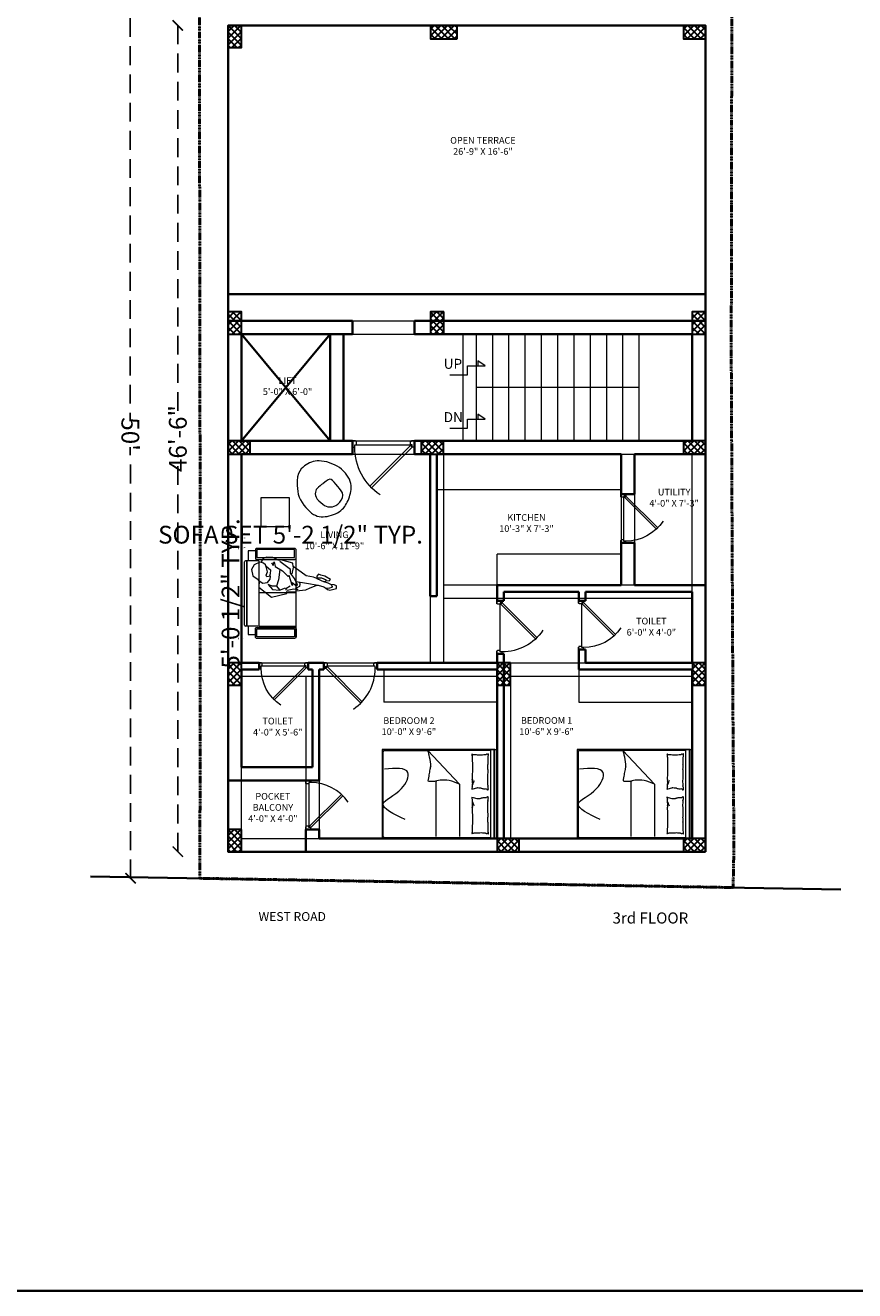
# Model space of a CAD drawing. Units: inches. Extents: x -16911 to -9621, y -48626 to -46270.
# Tile 15 of 20: x -10695 to -10135, y -48626 to -47771. Entities that reach past the tile are written whole.
import ezdxf

# ---------------------------------------------------------------- set-up
doc = ezdxf.new("R2010")
doc.units = ezdxf.units.IN
for name, pattern in [('DASHDOT', [1, 0.5, -0.25, 0, -0.25]), ('DASHED', [19.05, 12.7, -6.35]), ('DOT2', [3.175, 0, -3.175])]:
    doc.linetypes.add(name, pattern=pattern)
for name, color, linetype, lineweight in [('A-ANNO-DIMS', 2, 'Continuous', 13), ('A-ANNO-SYMB', 3, 'Continuous', 13), ('A-ANNO-TEXT', 7, 'Continuous', 18), ('A-AREA-IDEN', 3, 'Continuous', 18), ('A-DOOR', 4, 'Continuous', 18), ('A-FLOR-STRS', 3, 'Continuous', 18), ('A-FURN', 8, 'Continuous', 13), ('A-WALL', 7, 'Continuous', 35), ('C-PROP', 6, 'DASHDOT', 50), ('column', 12, 'Continuous', 30), ('DOOR', 143, 'Continuous', 9), ('EXT BEAM', 132, 'Continuous', 13), ('furniture', 35, 'Continuous', 15), ('Man', 8, 'Continuous', 5), ('S-BEAM', 132, 'Continuous', 25), ('S-COLS', 1, 'Continuous', 30), ('STAIRCASE', 137, 'Continuous', 5)]:
    doc.layers.add(name, color=color, linetype=linetype, lineweight=lineweight)
doc.styles.get("Standard").update_dxf_attribs({"font": 'swissel.ttf'})
doc.styles.add('style9', font='swisscl.ttf', dxfattribs={"height": 12})
doc.dimstyles.new('Dim9', dxfattribs={"dimtxt": 10, "dimasz": 0.199219, "dimexe": 1, "dimexo": 0.5, "dimgap": 1, "dimtad": 0, "dimdec": 1, "dimzin": 0, "dimdsep": 46, "dimlunit": 4, "dimtxsty": 'style9', "dimblk": 'ARCHTICK', "dimcen": 0.09, "dimclrd": 256, "dimclrt": 256, "dimadec": 0, "dimazin": 0, "dimtfac": 1, "dimtdec": 1, "dimtix": 1, "dimtofl": 0, "dimtmove": 1, "dimatfit": 3, "dimfxl": 9, "dimtolj": 1, "dimtzin": 0, "dimlwd": -1, "dimarcsym": 0})

# ---------------------------------------------------------------- blocks, each defined once
blk = doc.blocks.new('Bipman02')
blk.add_lwpolyline([(0.587, -0.067), (0.618, -0.05), (0.652, -0.054), (0.67, -0.038), (0.596, 0.007), (0.544, 0.016), (0.516, 0.03), (0.496, 0.007), (0.492, -0.023), (0.452, -0.006), (0.357, 0.011), (0.292, 0.055), (0.192, 0.129), (0.187, 0.172), (0.031, 0.216), (0.005, 0.207), (-0.069, 0.246), (-0.147, 0.25), (-0.195, 0.233), (-0.225, 0.181), (-0.238, 0.185), (-0.308, 0.15), (-0.343, 0.09), (-0.325, 0.011), (-0.256, -0.037), (-0.247, -0.058), (-0.251, -0.137), (-0.086, -0.263), (0.109, -0.215), (0.109, -0.193), (0.226, -0.197), (0.231, -0.184), (0.352, -0.171), (0.409, -0.145), (0.487, -0.115), (0.509, -0.11), (0.583, -0.132), (0.609, -0.15), (0.63, -0.164), (0.661, -0.176), (0.744, -0.154), (0.748, -0.119), (0.714, -0.105), (0.674, -0.102), (0.639, -0.084)], close=True)
for points in [[(-0.256, -0.045), (-0.199, -0.084), (-0.138, -0.076), (-0.104, -0.032), (-0.099, 0.007), (-0.147, -0.002), (-0.156, 0.016), (-0.138, 0.059), (-0.151, 0.111), (-0.165, 0.15), (-0.191, 0.172), (-0.217, 0.181)], [(-0.086, 0.177), (-0.065, 0.142), (-0.052, 0.19), (-0.039, 0.129), (0.053, 0.072), (0.127, 0.003), (0.135, 0.016), (0.174, -0.106), (0.187, -0.11), (0.179, -0.076), (0.235, -0.119), (0.248, -0.106), (0.209, -0.023), (0.157, 0.042), (0.157, 0.09), (0.018, 0.194)], [(-0.156, 0.133), (-0.099, 0.085), (-0.104, 0.033), (-0.112, 0.007)], [(0.018, 0.09), (0.001, -0.041), (-0.025, -0.123), (-0.078, -0.123), (-0.13, -0.102), (-0.073, -0.167), (0.014, -0.176), (0.092, -0.145), (0.101, -0.176)], [(0.192, 0.116), (0.174, 0.037)], [(-0.025, -0.123), (0.014, -0.171)], [(0.096, -0.154), (0.153, -0.119)], [(0.27, -0.076), (0.274, -0.097), (0.27, -0.128), (0.244, -0.141), (0.222, -0.145), (0.248, -0.163), (0.248, -0.171), (0.2, -0.163), (0.114, -0.18)], [(0.231, -0.063), (0.361, -0.084), (0.509, -0.109)], [(0.492, -0.023), (0.587, -0.067)], [(0.505, -0.015), (0.552, -0.015), (0.613, -0.041)], [(0.678, -0.11), (0.691, -0.128), (0.687, -0.141), (0.657, -0.15), (0.609, -0.154)]]:
    blk.add_lwpolyline(points)
blk = doc.blocks.new('erertety')
at = {"layer": 'furniture', "ltscale": 0.2}
for p, q in [((-17662.13, -45230.66), (-17662.13, -45176.69)), ((-17693.83, -45223.2), (-17693.83, -45184.43)), ((-17685.49, -45183.68), (-17693.08, -45183.68)), ((-17684.74, -45223.2), (-17684.74, -45184.43)), ((-17684.74, -45203.31), (-17662.13, -45203.31)), ((-17685.49, -45223.95), (-17693.08, -45223.95)), ((-17691.58, -45223.95), (-17691.58, -45229.1)), ((-17684.74, -45223.99), (-17662.13, -45223.99)), ((-17684.74, -45224.55), (-17662.13, -45224.55)), ((-17684.74, -45224.55), (-17662.13, -45224.55)), ((-17691.58, -45229.1), (-17687.09, -45229.1))]:
    blk.add_line(p, q, dxfattribs=at)
blk.add_lwpolyline([(-17687.09, -45177.54), (-17691.58, -45177.54), (-17691.58, -45183.68)], dxfattribs=at)
for points in [[(-17662.13, -45182.17), (-17662.13, -45176.97, 0.414214), (-17662.87, -45176.22), (-17686.34, -45176.22, 0.414214), (-17687.09, -45176.97), (-17687.09, -45182.17, 0.414214), (-17686.34, -45182.91), (-17662.87, -45182.91, 0.414214)], [(-17662.13, -45225.47), (-17662.13, -45230.66, -0.414214), (-17662.87, -45231.41), (-17686.34, -45231.41, -0.414214), (-17687.09, -45230.66), (-17687.09, -45225.47, -0.414214), (-17686.34, -45224.72), (-17662.87, -45224.72, -0.414214)]]:
    blk.add_lwpolyline(points, format="xyb", close=True, dxfattribs=at)
for points in [[(-17663.01, -45181.75), (-17663.01, -45176.82), (-17686.21, -45176.82), (-17686.21, -45181.75)], [(-17692.4, -45183.68), (-17692.4, -45223.95), (-17692.4, -45223.95), (-17692.4, -45183.68)], [(-17663.01, -45225.6), (-17663.01, -45230.53), (-17686.21, -45230.53), (-17686.21, -45225.6)]]:
    blk.add_lwpolyline(points, close=True, dxfattribs=at)
for centre, start, end in [((-17693.08, -45184.43), 90, 180), ((-17685.49, -45184.43), 0, 90), ((-17693.08, -45223.2), 180, 270), ((-17685.49, -45223.2), 270, 0)]:
    blk.add_arc(centre, 0.748, start, end, dxfattribs=at)
at = {"layer": 'furniture', "ltscale": 0.2, "xscale": 47.90818138957024, "yscale": 47.90818138957024, "zscale": 47.90818138957024}
blk.add_blockref('Bipman02', (-17673, -45193.44, 0), dxfattribs=at)
blk = doc.blocks.new('rthrty')
at = {"layer": 'furniture'}
blk.add_open_spline([(-17650.3, -45154.53), (-17651.97, -45142.9), (-17645.3, -45136.31), (-17637.11, -45132.37), (-17620.71, -45137.17), (-17612.47, -45149.45), (-17615.73, -45159.71), (-17619.67, -45168.02), (-17632.28, -45172.65), (-17641.84, -45170.43), (-17649.5, -45159.42), (-17650.3, -45154.53)], degree=3, dxfattribs=at)
at = {"layer": 'Man'}
blk.add_open_spline([(-17632.99, -45149.02), (-17629.89, -45146.6), (-17628, -45145.12), (-17623.29, -45151.15), (-17618.06, -45156.77), (-17623.15, -45164.08), (-17628.28, -45165.32), (-17631.61, -45164.6), (-17638.01, -45159.61), (-17638.81, -45154.69), (-17636.9, -45151.81), (-17632.99, -45149.02), (-17632.99, -45149.02)], degree=3, dxfattribs=at)
blk = doc.blocks.new('hjuyuiuyk')
at = {"layer": 'furniture'}
for p, q in [((-19327.49, -39738.98), (-19327.49, -39737.31)), ((-19327.49, -39737.31), (-19267.49, -39737.31, 0)), ((-19327.49, -39746.54), (-19327.49, -39737.31)), ((-19267.49, -39738.5), (-19327.49, -39738.5, 0)), ((-19327.49, -39738.5, 0), (-19327.49, -39814.72, 0)), ((-19327.49, -39738.5), (-19327.49, -39814.72)), ((-19267.49, -39738.5, 0), (-19327.49, -39738.5)), ((-19267.49, -39738.98, 0), (-19327.49, -39738.98)), ((-19268.1, -39741.33), (-19326.9, -39741.33)), ((-19326.9, -39741.33), (-19326.9, -39813.21)), ((-19268.1, -39813.21), (-19268.1, -39741.33)), ((-19267.49, -39737.31, 0), (-19267.49, -39738.98, 0)), ((-19267.49, -39746.54, 0), (-19267.49, -39737.31, 0)), ((-19267.49, -39814.72), (-19267.49, -39738.5)), ((-19267.49, -39814.72, 0), (-19267.49, -39738.5, 0)), ((-19300.88, -39753.22, 0), (-19301.49, -39750.81, 0)), ((-19294.97, -39753.22, 0), (-19294.37, -39750.81, 0)), ((-19300.67, -39754.09, 0), (-19300.88, -39753.22, 0)), ((-19295.19, -39754.09, 0), (-19294.97, -39753.22, 0)), ((-19304.07, -39762.52), (-19326.9, -39783.91)), ((-19304.07, -39762.52), (-19268.82, -39762.52)), ((-19326.9, -39813.21), (-19326.9, -39783.91)), ((-19268.82, -39778.34), (-19306.29, -39778.34)), ((-19327.49, -39814.72, 0), (-19267.49, -39814.72)), ((-19327.49, -39814.72), (-19267.49, -39814.72, 0)), ((-19269.1, -39814.21), (-19325.9, -39814.21)), ((-19325.9, -39814.21), (-19269.1, -39814.21))]:
    blk.add_line(p, q, dxfattribs=at)
for centre, radius, start, end in [((-19324.36, -39743.07, 0), 0.0997, 111.7883, 160.43603), ((-19324.39, -39743.06, 0), 0.0676, 160.43603, 281.89306), ((-19324.12, -39743.66, 0), 0.732, 94.30254, 111.7883), ((-19324.35, -39743.25, 0), 0.125, 21.9904, 101.89306), ((-19323.34, -39743.89, 0), 0.956, 158.57902, 188.13348), ((-19324.65, -39743.37, 0), 0.455, 338.57902, 21.9904), ((-19324.11, -39743.77, 0), 0.842, 59.34875, 94.30254), ((-19322.88, -39741.69, 0), 1.57, 239.34875, 264.74081), ((-19319.6, -39692.5, 0), 50.87, 266.13994, 268.60024), ((-19319.84, -39713.09, 0), 30.28, 268.09211, 271.28082), ((-19320.24, -39695.07, 0), 48.31, 271.28082, 273.40341), ((-19316.15, -39763.89, 0), 20.63, 90.1553, 93.40341), ((-19316.09, -39783.15, 0), 39.89, 86.99024, 90.1553), ((-19305.86, -39588.51, 0), 155.02, 266.99024, 268.59569), ((-19305.42, -39570.46, 0), 173.07, 268.59569, 270), ((-19305.42, -39718.38, 0), 25.15, 270, 273.68415), ((-19304.03, -39739.9, 0), 3.58, 273.68415, 287.19507), ((-19300.46, -39751.46, 0), 8.51, 98.43719, 107.19507), ((-19301.02, -39747.69, 0), 4.7, 90, 98.43719), ((-19301.12, -39743.14, 0), 0.997, 274.40021, 333.41948), ((-19301.02, -39745.63, 0), 2.64, 78.72762, 90), ((-19300.58, -39743.42, 0), 0.383, 333.41948, 78.72762), ((-19295.28, -39743.42, 0), 0.383, 101.27238, 206.58052), ((-19294.73, -39743.14, 0), 0.997, 206.58052, 265.59979), ((-19294.84, -39745.63, 0), 2.64, 90, 101.27238), ((-19294.84, -39747.69, 0), 4.7, 81.56281, 90), ((-19295.39, -39751.46, 0), 8.51, 72.80493, 81.56281), ((-19291.82, -39739.9, 0), 3.58, 252.80493, 266.31585), ((-19290.43, -39718.38, 0), 25.15, 266.31585, 270), ((-19290.43, -39570.46, 0), 173.07, 270, 271.40431), ((-19289.99, -39588.51, 0), 155.02, 271.40431, 273.00976), ((-19279.76, -39783.15, 0), 39.89, 89.8447, 93.00976), ((-19279.7, -39763.89, 0), 20.63, 86.59659, 89.8447), ((-19275.61, -39695.07, 0), 48.31, 266.59659, 268.71918), ((-19276.02, -39713.09, 0), 30.28, 268.71918, 271.90789), ((-19276.73, -39645.13, 0), 98.25, 271.00686, 272.7772), ((-19272.12, -39741.69, 0), 1.57, 275.25919, 300.65125), ((-19270.89, -39743.77, 0), 0.842, 85.69746, 120.65125), ((-19270.88, -39743.66, 0), 0.732, 68.2117, 85.69746), ((-19270.35, -39743.37, 0), 0.455, 158.0096, 201.42098), ((-19270.65, -39743.25, 0), 0.125, 78.10694, 158.0096), ((-19271.66, -39743.89, 0), 0.956, 351.86652, 21.42098), ((-19270.61, -39743.06, 0), 0.0676, 258.10694, 19.56397), ((-19270.64, -39743.07, 0), 0.0997, 19.56397, 68.2117), ((-19317.18, -39743.01, 0), 7.17, 188.13348, 192.10946), ((-19329.85, -39745.73, 0), 5.78, 7.6809, 12.10946), ((-19350.51, -39748.51, 0), 26.62, 3.36875, 7.6809), ((-19720.99, -39728.47, 0), 397.61, 356.49514, 356.94504), ((-19363.7, -39747.54, 0), 39.81, 356.94504, 358.36691), ((-19343.69, -39748.11, 0), 19.79, 358.36691, 3.36875), ((-19299.57, -39750.33, 0), 1.97, 177.33512, 194.04519), ((-19282.35, -39751.13, 0), 19.21, 171.99495, 177.33512), ((-19292.22, -39749.75, 0), 9.25, 167.80162, 171.99495), ((-19326.4, -39742.36, 0), 25.72, 347.80162, 350.31563), ((-19315.3, -39745.68, 0), 14.34, 360, 6.23236), ((-19306.91, -39745.68, 0), 5.95, 350.31563, 360), ((-19280.55, -39745.68, 0), 14.34, 173.76764, 180), ((-19288.94, -39745.68, 0), 5.95, 180, 189.68437), ((-19269.45, -39742.36, 0), 25.72, 189.68437, 192.19838), ((-19303.63, -39749.75, 0), 9.25, 8.00505, 12.19838), ((-19313.5, -39751.13, 0), 19.21, 2.66488, 8.00505), ((-19296.28, -39750.33, 0), 1.97, 345.95481, 2.66488), ((-19251.31, -39748.11, 0), 19.79, 176.63125, 181.63309), ((-19231.3, -39747.54, 0), 39.81, 181.63309, 183.05496), ((-19244.49, -39748.51, 0), 26.62, 172.3191, 176.63125), ((-18874.01, -39728.47, 0), 397.61, 183.05496, 183.50486), ((-19265.15, -39745.73, 0), 5.78, 167.89054, 172.3191), ((-19277.82, -39743.01, 0), 7.17, 347.89054, 351.86652), ((-19323.69, -39753.93, 0), 0.564, 170.00164, 196.69777), ((-19333.47, -39752.21, 0), 9.37, 350.00164, 356.49514), ((-19324.19, -39754.08, 0), 0.0385, 196.69777, 277.12039), ((-19324.51, -39751.59, 0), 2.55, 277.12039, 286.22115), ((-19324.42, -39751.9, 0), 2.23, 286.22115, 297.44392), ((-19322.81, -39754.99, 0), 1.25, 102.44799, 117.44392), ((-19322.32, -39757.22, 0), 3.54, 93.57397, 102.44799), ((-19318.44, -39837.61, 0), 84.03, 90.97549, 92.79548), ((-19315.55, -39952.16, 0), 198.61, 89.44614, 91.24735), ((-19314.9, -39885.06, 0), 131.51, 87.23256, 89.44614), ((-19310.57, -39795.48, 0), 41.81, 85.40123, 87.23256), ((-19304.32, -39717.78, 0), 36.14, 265.40123, 267.37117), ((-19297.32, -39733.09, 0), 21.54, 244.68893, 246.51559), ((-19305.66, -39747.05, 0), 6.83, 267.37117, 281.48268), ((-19297.32, -39733.09, 0), 21.54, 246.51559, 248.34226), ((-19297.32, -39733.09, 0), 21.54, 248.34226, 250.57202), ((-19297.32, -39733.09, 0), 21.54, 250.57202, 252.80178), ((-19303.46, -39757.91, 0), 4.25, 83.56595, 101.48268), ((-19303.37, -39757.16, 0), 3.49, 72.61359, 83.56595), ((-19300.33, -39747.43, 0), 6.7, 252.61359, 260.5159), ((-19300.13, -39746.25, 0), 7.9, 260.5159, 265.91706), ((-19300.69, -39754.1, 0), 0.0267, 265.91706, 14.04494), ((-19295.16, -39754.1, 0), 0.0267, 165.95506, 274.08294), ((-19295.72, -39746.25, 0), 7.9, 274.08294, 279.4841), ((-19295.52, -39747.43, 0), 6.7, 279.4841, 287.38641), ((-19292.48, -39757.16, 0), 3.49, 96.43405, 107.38641), ((-19292.39, -39757.91, 0), 4.25, 78.51732, 96.43405), ((-19298.54, -39733.09, 0), 21.54, 287.19822, 289.42798), ((-19290.19, -39747.05, 0), 6.83, 258.51732, 272.62883), ((-19298.54, -39733.09, 0), 21.54, 289.42798, 291.65774), ((-19298.54, -39733.09, 0), 21.54, 291.65774, 293.48441), ((-19298.54, -39733.09, 0), 21.54, 293.48441, 295.31107), ((-19291.53, -39717.78, 0), 36.14, 272.62883, 274.59877), ((-19285.28, -39795.48, 0), 41.81, 92.76744, 94.59877), ((-19280.95, -39885.06, 0), 131.51, 90.55386, 92.76744), ((-19280.3, -39952.16, 0), 198.61, 88.75265, 90.55386), ((-19277.1, -39805.01, 0), 51.42, 86.42603, 88.75265), ((-19274.68, -39799.75, 0), 46.07, 86.55746, 89.01709), ((-19272.19, -39754.99, 0), 1.25, 62.55608, 77.55201), ((-19270.58, -39751.9, 0), 2.23, 242.55608, 253.77885), ((-19270.49, -39751.59, 0), 2.55, 253.77885, 262.87961), ((-19261.53, -39752.21, 0), 9.37, 183.50486, 189.99836), ((-19270.81, -39754.08, 0), 0.0385, 262.87961, 343.30223), ((-19271.31, -39753.93, 0), 0.564, 343.30223, 9.99836), ((-19279.47, -39774.89), 27.53, 153.30845, 168.74227), ((-19287.94, -39773.2), 18.89, 168.74227, 187.39945), ((-19242.78, -39767.34), 64.43, 187.39945, 189.27191), ((-19333.07, -39782.08), 27.05, 6.38169, 9.27191), ((-19306.77, -39846.83), 66.07, 105.93519, 107.73639), ((-19318.41, -39806.06), 23.67, 102.92554, 105.93519), ((-19287.64, -39956.87), 177.57, 99.72434, 101.71957), ((-19317.24, -39783.9), 2.09, 82.26962, 100.72756), ((-19317.9, -39788.76), 6.99, 76.8096, 82.26962), ((-19295.64, -39693.77), 90.57, 256.8096, 258.32586), ((-19295.11, -39691.23), 93.17, 258.32586, 260.50498), ((-19288.03, -39648.9), 136.08, 260.50498, 262.308), ((-19336.71, -39780.62), 30.63, 354.11415, 359.23133), ((-19321.79, -39780.82), 15.7, 359.23133, 6.38169), ((-19325.9, -39813.21), 1, 180, 270), ((-19269.1, -39813.21), 1, 270, 0)]:
    blk.add_arc(centre, radius, start, end, dxfattribs=at)
blk.add_open_spline([(-19280.24, -39799.21), (-19283.87, -39806.94), (-19290.73, -39821.55), (-19298.08, -39801.09), (-19315.85, -39793.47), (-19314.86, -39805.92), (-19314.29, -39813.13)], degree=3, knots=[0, 0, 0, 0, 18.167809, 34.338432, 45.972904, 61.997799, 61.997799, 61.997799, 61.997799], dxfattribs=at)
blk = doc.blocks.new('A$C1C9D3E54')
at = {"layer": 'DOOR'}
blk.add_line((18676.53, 5780.72), (18710.53, 5780.72), dxfattribs=at)
blk.add_lwpolyline([(18685.01, 5806.62), (18710.47, 5781.16), (18711.53, 5782.22), (18686.07, 5807.68), (18685.01, 5806.62)], dxfattribs=at)
blk.add_lwpolyline([(18674.03, 5778.22), (18676.03, 5778.22), (18674.03, 5778.22), (18674.03, 5782.22), (18675.53, 5782.22), (18675.53, 5780.72), (18676.53, 5780.72), (18676.53, 5778.72), (18676.41, 5778.72), (18676.41, 5778.6, -0.414214), (18676.16, 5778.35), (18676.03, 5778.35), (18676.03, 5778.22)], format="xyb", dxfattribs=at)
blk.add_lwpolyline([(18713.03, 5782.22), (18711.53, 5782.22), (18711.53, 5780.72), (18710.53, 5780.72), (18710.53, 5778.72), (18710.66, 5778.72), (18710.66, 5778.6, 0.414214), (18710.91, 5778.35), (18711.03, 5778.35), (18711.03, 5778.22), (18713.03, 5778.22), (18711.03, 5778.22), (18713.03, 5778.22), (18713.03, 5782.22)], format="xyb", close=True, dxfattribs=at)
blk.add_arc((18711.53, 5782.22), 36, 124.03362, 180, dxfattribs=at)
blk = doc.blocks.new('_ArchTick')
at = {"color": 0, "linetype": 'ByBlock', "const_width": 0.15}
blk.add_lwpolyline([(-0.5, -0.5), (0.5, 0.5)], dxfattribs=at)
blk = doc.blocks.new('*D24')
at = {"layer": 'A-ANNO-DIMS', "color": 0, "linetype": 'DOT2', "lineweight": -2, "transparency": 16777216}
for p, q in [((-10623.85, -47747.46), (-10625.04, -47747.46)), ((-10623.49, -48347.46), (-10624.67, -48347.46))]:
    blk.add_line(p, q, dxfattribs=at)
at = {"layer": 'A-ANNO-DIMS', "color": 0, "linetype": 'DASHED', "lineweight": 25, "transparency": 16777216}
for p, q in [((-10624.04, -47747.46), (-10623.86, -48038.62)), ((-10623.67, -48347.46), (-10623.85, -48056.3))]:
    blk.add_line(p, q, dxfattribs=at)
at = {"layer": 'Defpoints', "color": 0, "transparency": 16777216}
for p in [(-10624.04, -47747.46), (-10605.22, -47747.45), (-10604.86, -48347.45)]:
    blk.add_point(p, dxfattribs=at)
at = {"layer": 'A-ANNO-DIMS', "color": 0, "lineweight": 25, "transparency": 16777216, "xscale": 7, "yscale": 7, "zscale": 7}
for p, rotation in [((-10624.04, -47747.46), 90.0346840750536), ((-10623.67, -48347.46), 270.0346840750536)]:
    blk.add_blockref('_ArchTick', p, dxfattribs=dict(at, rotation=rotation))
at = {"layer": 'A-ANNO-DIMS', "color": 0, "transparency": 16777216, "insert": (-10623.85, -48047.46), "char_height": 12, "attachment_point": 5, "rotation": 270.03468, "style": 'style9'}
blk.add_mtext("\\A1;50'", dxfattribs=at)
blk = doc.blocks.new('*D26')
at = {"layer": 'A-ANNO-DIMS', "color": 0, "linetype": 'DOT2', "lineweight": -2, "transparency": 16777216}
for p, q in [((-10591.56, -47771.49), (-10592.75, -47771.49)), ((-10591.56, -48329.45), (-10592.75, -48329.45))]:
    blk.add_line(p, q, dxfattribs=at)
at = {"layer": 'A-ANNO-DIMS', "color": 0, "linetype": 'DASHED', "lineweight": 25, "transparency": 16777216}
for p, q in [((-10591.75, -47771.49), (-10591.75, -48032.84)), ((-10591.75, -48329.45), (-10591.75, -48068.11))]:
    blk.add_line(p, q, dxfattribs=at)
at = {"layer": 'Defpoints', "color": 0, "transparency": 16777216}
for p in [(-10557.82, -47771.49), (-10591.75, -48329.45), (-10557.82, -48329.45)]:
    blk.add_point(p, dxfattribs=at)
at = {"layer": 'A-ANNO-DIMS', "color": 0, "lineweight": 25, "transparency": 16777216, "xscale": 7, "yscale": 7, "zscale": 7}
for p, rotation in [((-10591.75, -47771.49), 90), ((-10591.75, -48329.45), 270)]:
    blk.add_blockref('_ArchTick', p, dxfattribs=dict(at, rotation=rotation))
at = {"layer": 'A-ANNO-DIMS', "color": 0, "transparency": 16777216, "insert": (-10591.75, -48050.47), "char_height": 12, "attachment_point": 5, "rotation": 90, "style": 'style9'}
blk.add_mtext('\\A1;46\'-6"', dxfattribs=at)
blk = doc.blocks.new('THYHYTJ')
at = {"layer": 'STAIRCASE', "ltscale": 10}
for p, q in [((-7981.18, -46346.18), (-7984.62, -46351.1)), ((-7981.18, -46358.18), (-7981.18, -46346.18)), ((-7984.62, -46351.1), (-7981.18, -46351.1)), ((-7975.18, -46358.18), (-7981.18, -46358.18)), ((-7975.18, -46370.18), (-7975.18, -46358.18))]:
    blk.add_line(p, q, dxfattribs=at)
blk = doc.blocks.new('COLUMNS')
at = {"layer": 'column'}
h = blk.add_hatch(dxfattribs=at)
h.set_pattern_fill('ANSI37', color=256, angle=-720)
h.set_pattern_definition([(45, (21703.4588, -104481.6704), (-2.24506403, 2.24506403), []), (135, (21703.4588, -104481.6704), (-2.24506403, -2.24506403), [])])
h.paths.add_polyline_path([(-12061.47, -46401.86), (-12052.47, -46401.86), (-12052.47, -46386.86), (-12061.47, -46386.86)])
h = blk.add_hatch(dxfattribs=at)
h.set_pattern_fill('ANSI37', color=256, angle=-810)
h.set_pattern_definition([(315, (-70004.5392, -80151.7886), (2.24506403, 2.24506403), []), (45, (-70004.5392, -80151.7886), (-2.24506403, 2.24506403), [])])
h.paths.add_polyline_path([(-11924.72, -46386.86), (-11924.72, -46395.86), (-11906.72, -46395.86), (-11906.72, -46386.86)])
h = blk.add_hatch(dxfattribs=at)
h.set_pattern_fill('ANSI37', color=256, angle=-810)
h.set_pattern_definition([(315, (-69833.7395, -80151.7886), (2.24506403, 2.24506403), []), (45, (-69833.7395, -80151.7886), (-2.24506403, 2.24506403), [])])
h.paths.add_polyline_path([(-11753.92, -46386.86), (-11753.92, -46395.86), (-11738.92, -46395.86), (-11738.92, -46386.86)])
h = blk.add_hatch(dxfattribs=at)
h.set_pattern_fill('ANSI37', color=256, angle=-900)
h.set_pattern_definition([(225, (-45817.4075, 11499.4594), (2.24506403, -2.24506403), []), (315, (-45817.4075, 11499.4594), (2.24506403, 2.24506403), [])])
h.paths.add_polyline_path([(-12052.47, -46580.36), (-12061.47, -46580.36), (-12061.47, -46595.36), (-12052.47, -46595.36)])
h = blk.add_hatch(dxfattribs=at)
h.set_pattern_fill('ANSI37', color=256, angle=-720)
h.set_pattern_definition([(45, (21840.2088, -104675.1704), (-2.24506403, 2.24506403), []), (135, (21840.2088, -104675.1704), (-2.24506403, -2.24506403), [])])
h.paths.add_polyline_path([(-11924.72, -46595.36), (-11915.72, -46595.36), (-11915.72, -46580.36), (-11924.72, -46580.36)])
h = blk.add_hatch(dxfattribs=at)
h.set_pattern_fill('ANSI37', color=256, angle=-900)
h.set_pattern_definition([(225, (-45503.8578, 11499.4594), (2.24506403, -2.24506403), []), (315, (-45503.8578, 11499.4594), (2.24506403, 2.24506403), [])])
h.paths.add_polyline_path([(-11738.92, -46580.36), (-11747.92, -46580.36), (-11747.92, -46595.36), (-11738.92, -46595.36)])
h = blk.add_hatch(dxfattribs=at)
h.set_pattern_fill('ANSI37', color=256, angle=-810)
h.set_pattern_definition([(315, (-70141.2892, -80432.2886), (2.24506403, 2.24506403), []), (45, (-70141.2892, -80432.2886), (-2.24506403, 2.24506403), [])])
h.paths.add_polyline_path([(-12061.47, -46667.36), (-12061.47, -46676.36), (-12046.47, -46676.36), (-12046.47, -46667.36)])
h = blk.add_hatch(dxfattribs=at)
h.set_pattern_fill('ANSI37', color=256, angle=-810)
h.set_pattern_definition([(315, (-70010.7892, -80432.2886), (2.24506403, 2.24506403), []), (45, (-70010.7892, -80432.2886), (-2.24506403, 2.24506403), [])])
h.paths.add_polyline_path([(-11930.97, -46667.36), (-11930.97, -46676.36), (-11915.97, -46676.36), (-11915.97, -46667.36)])
h = blk.add_hatch(dxfattribs=at)
h.set_pattern_fill('ANSI37', color=256, angle=-810)
h.set_pattern_definition([(315, (-69833.7395, -80432.2886), (2.24506403, 2.24506403), []), (45, (-69833.7395, -80432.2886), (-2.24506403, 2.24506403), [])])
h.paths.add_polyline_path([(-11753.92, -46667.36), (-11753.92, -46676.36), (-11738.92, -46676.36), (-11738.92, -46667.36)])
h = blk.add_hatch(dxfattribs=at)
h.set_pattern_fill('ANSI37', color=256, angle=-540)
h.set_pattern_definition([(225, (-45817.4075, 11262.5055), (2.24506403, -2.24506403), []), (315, (-45817.4075, 11262.5055), (2.24506403, 2.24506403), [])])
h.paths.add_polyline_path([(-12052.47, -46817.31), (-12061.47, -46817.31), (-12061.47, -46832.31), (-12052.47, -46832.31)])
h = blk.add_hatch(dxfattribs=at)
h.set_pattern_fill('ANSI37', color=256, angle=-720)
h.set_pattern_definition([(45, (21885.2088, -104912.1242), (-2.24506403, 2.24506403), []), (135, (21885.2088, -104912.1242), (-2.24506403, -2.24506403), [])])
h.paths.add_polyline_path([(-11879.72, -46832.31), (-11870.72, -46832.31), (-11870.72, -46817.31), (-11879.72, -46817.31)])
h = blk.add_hatch(dxfattribs=at)
h.set_pattern_fill('ANSI37', color=256, angle=-720)
h.set_pattern_definition([(45, (22017.1023, -104912.1242), (-2.24506403, 2.24506403), []), (135, (22017.1023, -104912.1242), (-2.24506403, -2.24506403), [])])
h.paths.add_polyline_path([(-11747.83, -46832.31), (-11738.83, -46832.31), (-11738.83, -46817.31), (-11747.83, -46817.31)])
h = blk.add_hatch(dxfattribs=at)
h.set_pattern_fill('ANSI37', color=256, angle=-720)
h.set_pattern_definition([(45, (21703.4588, -105024.6242), (-2.24506403, 2.24506403), []), (135, (21703.4588, -105024.6242), (-2.24506403, -2.24506403), [])])
h.paths.add_polyline_path([(-12061.47, -46944.81), (-12052.47, -46944.81), (-12052.47, -46929.81), (-12061.47, -46929.81)])
h = blk.add_hatch(dxfattribs=at)
h.set_pattern_fill('ANSI37', color=256, angle=-810)
h.set_pattern_definition([(315, (-69959.5392, -80700.7425), (2.24506403, 2.24506403), []), (45, (-69959.5392, -80700.7425), (-2.24506403, 2.24506403), [])])
h.paths.add_polyline_path([(-11879.72, -46935.81), (-11879.72, -46944.81), (-11864.72, -46944.81), (-11864.72, -46935.81)])
h = blk.add_hatch(dxfattribs=at)
h.set_pattern_fill('ANSI37', color=256, angle=-810)
h.set_pattern_definition([(315, (-69833.7395, -80700.7425), (2.24506403, 2.24506403), []), (45, (-69833.7395, -80700.7425), (-2.24506403, 2.24506403), [])])
h.paths.add_polyline_path([(-11753.92, -46935.81), (-11753.92, -46944.81), (-11738.92, -46944.81), (-11738.92, -46935.81)])
at = {"layer": 'column', "ltscale": 0.05}
for points in [[(-12052.47, -46386.86), (-12061.47, -46386.86), (-12061.47, -46401.86), (-12052.47, -46401.86)], [(-11906.72, -46395.86), (-11906.72, -46386.86), (-11924.72, -46386.86), (-11924.72, -46395.86)], [(-11738.92, -46395.86), (-11738.92, -46386.86), (-11753.92, -46386.86), (-11753.92, -46395.86)], [(-12061.47, -46595.36), (-12052.47, -46595.36), (-12052.47, -46580.36), (-12061.47, -46580.36)], [(-11915.72, -46580.36), (-11924.72, -46580.36), (-11924.72, -46595.36), (-11915.72, -46595.36)], [(-11747.92, -46595.36), (-11738.92, -46595.36), (-11738.92, -46580.36), (-11747.92, -46580.36)], [(-12046.47, -46676.36), (-12046.47, -46667.36), (-12061.47, -46667.36), (-12061.47, -46676.36)], [(-11915.97, -46676.36), (-11915.97, -46667.36), (-11930.97, -46667.36), (-11930.97, -46676.36)], [(-11738.92, -46676.36), (-11738.92, -46667.36), (-11753.92, -46667.36), (-11753.92, -46676.36)], [(-12061.47, -46832.31), (-12052.47, -46832.31), (-12052.47, -46817.31), (-12061.47, -46817.31)], [(-11870.72, -46817.31), (-11879.72, -46817.31), (-11879.72, -46832.31), (-11870.72, -46832.31)], [(-11738.83, -46817.31), (-11747.83, -46817.31), (-11747.83, -46832.31), (-11738.83, -46832.31)], [(-12052.47, -46929.81), (-12061.47, -46929.81), (-12061.47, -46944.81), (-12052.47, -46944.81)], [(-11864.72, -46944.81), (-11864.72, -46935.81), (-11879.72, -46935.81), (-11879.72, -46944.81)], [(-11738.92, -46944.81), (-11738.92, -46935.81), (-11753.92, -46935.81), (-11753.92, -46944.81)]]:
    blk.add_lwpolyline(points, close=True, dxfattribs=at)
blk = doc.blocks.new('3RD ROOF BEAMS')
at = {"layer": 'EXT BEAM'}
for p, q in [((-11461.47, -46586.36), (-11324.72, -46586.36)), ((-11461.47, -46944.81), (-11461.47, -46586.36)), ((-11320.47, -46586.36), (-11138.92, -46586.36)), ((-11138.92, -46944.81), (-11138.92, -46586.36)), ((-11452.47, -46595.36), (-11324.72, -46595.36)), ((-11392.47, -46595.36), (-11392.47, -46667.36)), ((-11383.47, -46595.36), (-11383.47, -46667.36)), ((-11320.47, -46595.36), (-11147.92, -46595.36)), ((-11302.92, -46595.36), (-11302.92, -46667.36)), ((-11293.92, -46595.36), (-11293.92, -46667.36)), ((-11147.92, -46667.36), (-11147.92, -46595.36)), ((-11446.47, -46667.36), (-11335.47, -46667.36)), ((-11320.47, -46667.36), (-11138.92, -46667.36)), ((-11452.47, -46817.31), (-11452.47, -46676.36)), ((-11446.47, -46676.36), (-11335.47, -46676.36)), ((-11324.97, -46676.36), (-11324.97, -46817.31)), ((-11320.47, -46676.36), (-11138.92, -46676.36)), ((-11315.97, -46676.36), (-11315.97, -46817.31)), ((-11195.92, -46676.36), (-11195.92, -46764.81)), ((-11186.92, -46676.36), (-11186.92, -46764.81)), ((-11147.92, -46817.31), (-11147.92, -46676.36)), ((-11147.92, -46764.81), (-11315.97, -46764.81)), ((-11147.92, -46773.81), (-11315.97, -46773.81)), ((-11452.47, -46817.31), (-11147.92, -46817.31)), ((-11452.47, -46826.31), (-11279.72, -46826.31)), ((-11452.47, -46944.81), (-11452.47, -46826.31)), ((-11408.97, -46826.31), (-11408.97, -46935.81)), ((-11399.97, -46826.31), (-11399.97, -46935.81)), ((-11279.72, -46826.31), (-11279.72, -46935.81)), ((-11270.72, -46826.31), (-11147.92, -46826.31)), ((-11270.72, -46826.31), (-11270.72, -46935.81)), ((-11147.92, -46935.81), (-11147.92, -46826.31)), ((-11452.47, -46935.81), (-11279.72, -46935.81)), ((-11270.72, -46935.81), (-11147.92, -46935.81)), ((-11461.47, -46944.81), (-11138.92, -46944.81))]:
    blk.add_line(p, q, dxfattribs=at)
blk = doc.blocks.new('*D73')
at = {"layer": 'A-ANNO-DIMS', "linetype": 'DASHED', "transparency": 16777216}
for p, q in [((-10546.8, -48115.39), (-10547, -48115.39)), ((-10484.48, -48115.39), (-10484.28, -48115.39))]:
    blk.add_line(p, q, dxfattribs=at)
at = {"layer": 'A-ANNO-DIMS', "color": 0, "linetype": 'DOT2', "lineweight": -2, "transparency": 16777216}
for p, q in [((-10546.8, -48124.24), (-10546.8, -48114.39)), ((-10484.48, -48124.24), (-10484.48, -48114.39))]:
    blk.add_line(p, q, dxfattribs=at)
at = {"layer": 'Defpoints', "color": 0, "transparency": 16777216}
for p in [(-10484.48, -48115.39), (-10546.8, -48124.74), (-10484.48, -48124.74)]:
    blk.add_point(p, dxfattribs=at)
at = {"layer": 'A-ANNO-DIMS', "transparency": 16777216, "xscale": 0.19921875, "yscale": 0.19921875, "zscale": 0.19921875}
blk.add_blockref('_ArchTick', (-10546.8, -48115.39), dxfattribs=at)
at = {"layer": 'A-ANNO-DIMS', "transparency": 16777216, "xscale": 0.19921875, "yscale": 0.19921875, "zscale": 0.19921875, "rotation": 180}
blk.add_blockref('_ArchTick', (-10484.48, -48115.39), dxfattribs=at)
at = {"layer": 'A-ANNO-DIMS', "transparency": 16777216, "insert": (-10515.64, -48115.39), "char_height": 12, "attachment_point": 5, "style": 'style9'}
blk.add_mtext('\\A1;SOFA SET 5\'-2 1/2" TYP.', dxfattribs=at)
blk = doc.blocks.new('*D74')
at = {"layer": 'A-ANNO-DIMS', "color": 0, "linetype": 'DOT2', "lineweight": -2, "transparency": 16777216}
for p, q in [((-10547.3, -48124.74), (-10557.15, -48124.74)), ((-10547.3, -48185.44), (-10557.15, -48185.44))]:
    blk.add_line(p, q, dxfattribs=at)
at = {"layer": 'A-ANNO-DIMS', "linetype": 'DASHED', "transparency": 16777216}
for p, q in [((-10556.15, -48124.74), (-10556.15, -48124.54)), ((-10556.15, -48185.44), (-10556.15, -48185.64))]:
    blk.add_line(p, q, dxfattribs=at)
at = {"layer": 'Defpoints', "color": 0, "transparency": 16777216}
for p in [(-10556.15, -48124.74), (-10546.8, -48124.74), (-10546.8, -48185.44)]:
    blk.add_point(p, dxfattribs=at)
at = {"layer": 'A-ANNO-DIMS', "transparency": 16777216, "xscale": 0.19921875, "yscale": 0.19921875, "zscale": 0.19921875}
for p, rotation in [((-10556.15, -48124.74), 270), ((-10556.15, -48185.44), 90)]:
    blk.add_blockref('_ArchTick', p, dxfattribs=dict(at, rotation=rotation))
at = {"layer": 'A-ANNO-DIMS', "transparency": 16777216, "insert": (-10556.15, -48155.09), "char_height": 12, "attachment_point": 5, "rotation": 90, "style": 'style9'}
blk.add_mtext('\\A1;5\'-0 1/2" TYP.', dxfattribs=at)

msp = doc.modelspace()

# ---------------------------------------------------------------- linework, layer by layer
at = {"layer": 'A-FLOR-STRS', "ltscale": 10}
for p, q in [((-10390.274, -47979.994), (-10390.274, -48051.994)), ((-10379.274, -47979.994), (-10379.274, -48051.994)), ((-10368.274, -47979.994), (-10368.274, -48051.994)), ((-10357.274, -47979.994), (-10357.274, -48051.994)), ((-10346.274, -47979.994), (-10346.274, -48051.994)), ((-10335.274, -47979.994), (-10335.274, -48051.994)), ((-10324.274, -47979.994), (-10324.274, -48051.994)), ((-10313.274, -47979.994), (-10313.274, -48051.994)), ((-10302.274, -47979.994), (-10302.274, -48051.994)), ((-10291.274, -47979.994), (-10291.274, -48051.994)), ((-10280.274, -47979.994), (-10280.274, -48051.994)), ((-10280.274, -48015.994), (-10390.274, -48015.994))]:
    msp.add_line(p, q, dxfattribs=at)
at = {"layer": 'A-FURN', "ltscale": 0.2}
for p, q in [((-10292.274, -48084.994), (-10416.824, -48084.994)), ((-10292.274, -48128.448), (-10376.074, -48128.448)), ((-10376.074, -48149.448), (-10376.074, -48128.448)), ((-10452.574, -48206.448, 0), (-10452.574, -48228.448, 0)), ((-10320.774, -48206.448), (-10320.774, -48228.448)), ((-10376.074, -48228.448), (-10452.574, -48228.448)), ((-10320.774, -48228.448), (-10244.274, -48228.448))]:
    msp.add_line(p, q, dxfattribs=at)
at = {"layer": 'A-FURN'}
msp.add_lwpolyline([(-10516.228, -48090.39), (-10535.588, -48090.39), (-10535.588, -48109.75), (-10516.228, -48109.75)], close=True, dxfattribs=at)
at = {"layer": 'A-WALL'}
for p, q in [((-10235.274, -47771.494), (-10557.824, -47771.494)), ((-10557.824, -47970.994), (-10557.824, -47771.494)), ((-10235.274, -47771.494), (-10235.274, -47970.994)), ((-10557.824, -47952.994), (-10235.274, -47952.994)), ((-10557.824, -48281.448), (-10557.824, -47970.994)), ((-10473.824, -47970.994), (-10557.824, -47970.994)), ((-10473.824, -47979.994), (-10473.824, -47970.994)), ((-10235.274, -47970.994), (-10431.824, -47970.994)), ((-10431.824, -47979.994), (-10431.824, -47970.994)), ((-10235.274, -47970.994), (-10235.274, -48060.994)), ((-10548.824, -48051.994), (-10548.824, -47979.994)), ((-10473.824, -47979.994), (-10548.824, -47979.994)), ((-10548.824, -47979.994), (-10488.824, -48051.994)), ((-10548.824, -48051.994), (-10488.824, -47979.994)), ((-10488.824, -48051.994), (-10488.824, -47979.994)), ((-10479.824, -48051.994), (-10479.824, -47979.994)), ((-10244.274, -47979.994), (-10431.824, -47979.994)), ((-10244.274, -47979.994), (-10244.274, -48051.994)), ((-10473.824, -48051.994), (-10548.824, -48051.994)), ((-10473.824, -48060.994), (-10473.824, -48051.994)), ((-10244.274, -48051.994), (-10431.824, -48051.994)), ((-10431.824, -48060.994), (-10431.824, -48051.994)), ((-10548.824, -48201.948), (-10548.824, -48060.994)), ((-10473.824, -48060.994), (-10548.824, -48060.994)), ((-10421.324, -48060.994), (-10431.824, -48060.994)), ((-10421.324, -48060.994), (-10421.324, -48156.994)), ((-10292.274, -48060.994), (-10416.824, -48060.994)), ((-10416.824, -48060.994), (-10416.824, -48156.994)), ((-10292.274, -48060.994), (-10292.274, -48087.994)), ((-10235.274, -48060.994), (-10283.274, -48060.994)), ((-10283.274, -48060.994), (-10283.274, -48087.994)), ((-10235.274, -48060.994), (-10235.274, -48149.448)), ((-10292.274, -48087.994), (-10283.274, -48087.994)), ((-10292.274, -48120.994), (-10292.274, -48149.448)), ((-10292.274, -48120.994), (-10283.274, -48120.994)), ((-10283.274, -48120.994), (-10283.274, -48149.448)), ((-10376.074, -48159.948), (-10376.074, -48149.448)), ((-10376.074, -48149.448), (-10292.274, -48149.448)), ((-10283.274, -48149.448), (-10235.274, -48149.448)), ((-10235.274, -48149.448), (-10235.274, -48329.448)), ((-10416.824, -48156.994), (-10421.324, -48156.994)), ((-10376.074, -48159.948), (-10371.574, -48159.948)), ((-10371.574, -48159.948), (-10371.574, -48153.948)), ((-10371.574, -48153.948), (-10320.774, -48153.948)), ((-10320.774, -48153.948), (-10320.774, -48159.948)), ((-10320.774, -48159.948), (-10316.274, -48159.948)), ((-10316.274, -48153.948), (-10316.274, -48159.948)), ((-10316.274, -48153.948), (-10244.274, -48153.948)), ((-10244.274, -48153.948), (-10244.274, -48201.948)), ((-10320.774, -48192.948), (-10320.774, -48206.448)), ((-10320.774, -48192.948), (-10316.274, -48192.948)), ((-10316.274, -48192.948), (-10316.274, -48201.948)), ((-10548.824, -48201.948), (-10536.824, -48201.948)), ((-10536.824, -48201.948), (-10536.824, -48206.448)), ((-10503.824, -48201.948), (-10493.074, -48201.948)), ((-10503.824, -48201.948), (-10503.824, -48206.448)), ((-10493.074, -48206.448), (-10493.074, -48201.948)), ((-10457.074, -48201.948), (-10376.074, -48201.948)), ((-10457.074, -48206.448), (-10457.074, -48201.948)), ((-10376.074, -48201.948), (-10376.074, -48195.948)), ((-10376.074, -48195.948), (-10371.574, -48195.948)), ((-10371.574, -48320.448), (-10371.574, -48195.948)), ((-10316.274, -48201.948), (-10244.274, -48201.948)), ((-10548.824, -48272.448), (-10548.824, -48206.448)), ((-10548.824, -48206.448), (-10536.824, -48206.448)), ((-10503.824, -48206.448), (-10500.824, -48206.448)), ((-10500.824, -48272.448), (-10500.824, -48206.448)), ((-10496.324, -48281.448), (-10496.324, -48206.448)), ((-10496.324, -48206.448), (-10493.074, -48206.448)), ((-10457.074, -48206.448), (-10376.074, -48206.448)), ((-10376.074, -48320.448), (-10376.074, -48206.448)), ((-10320.774, -48206.448), (-10244.274, -48206.448)), ((-10244.274, -48206.448), (-10244.274, -48320.448)), ((-10548.824, -48272.448), (-10500.824, -48272.448)), ((-10557.824, -48329.448), (-10557.824, -48281.448)), ((-10557.824, -48281.448), (-10496.324, -48281.448)), ((-10505.324, -48329.448), (-10505.324, -48314.448)), ((-10505.324, -48314.448), (-10496.324, -48314.448)), ((-10496.324, -48320.448), (-10496.324, -48314.448)), ((-10496.324, -48320.448), (-10376.074, -48320.448)), ((-10371.574, -48320.448), (-10244.274, -48320.448)), ((-10557.824, -48329.448), (-10505.324, -48329.448)), ((-10505.324, -48329.448), (-10235.274, -48329.448)), ((-10143.897, -48354.931), (-10650.699, -48346.171))]:
    msp.add_line(p, q, dxfattribs=at)
msp.add_lwpolyline([(-13429.245, -47344.007), (-9756.987, -47344.007), (-9756.987, -48625.922), (-13429.245, -48625.922)], close=True, dxfattribs=at)
at = {"layer": 'C-PROP'}
msp.add_lwpolyline([(-10576.824, -48347.448), (-10216.642, -48353.673), (-10216.081, -48325.085), (-10216.744, -48240.245), (-10217.91, -47994.15), (-10217.524, -47752.494), (-10577.187, -47747.449), (-10576.649, -48147.594)], close=True, dxfattribs=at)

# ---------------------------------------------------------------- block references
at = {"layer": 'A-ANNO-SYMB', "rotation": 270.0000000000144}
for p in [(35962.08, -55982.596), (35962.08, -56018.596)]:
    msp.add_blockref('THYHYTJ', p, dxfattribs=at)
at = {"layer": 'A-DOOR'}
for p, xscale, yscale, zscale, rotation in [((-30584.318, -41829.291), -1.076923076922859, 1.076923076922859, 1.076923076922859, 180), ((-15181.791, -63922.097), -0.8461538461538624, 0.8461538461538624, 0.8461538461538624, 270), ((-15710.069, -65433.515), -0.9230769230769229, 0.9230769230769229, 0.9230769230769229, 270), ((-15210.291, -63994.051), -0.8461538461538624, 0.8461538461538624, 0.8461538461538624, 270), ((-26337.927, -43312.682), -0.8461538461538624, 0.8461538461538624, 0.8461538461538624, 180), ((6780.493, -42868.203), 0.9230769230769229, 0.9230769230769229, 0.9230769230769229, 180), ((-15394.59, -32480.345), 0.8461538461538624, 0.8461538461538624, 0.8461538461538624, 270)]:
    msp.add_blockref('A$C1C9D3E54', p, dxfattribs=dict(at, xscale=xscale, yscale=yscale, zscale=zscale, rotation=rotation))
at = {"layer": 'A-FURN'}
msp.add_blockref('rthrty', (7139.502, -2931.691), dxfattribs=at)
at = {"layer": 'A-FURN', "xscale": 1.1, "yscale": 1.1, "zscale": 1.1}
msp.add_blockref('erertety', (8916.41, 1569.111, 0), dxfattribs=at)
at = {"layer": 'A-FURN', "rotation": 270}
for p in [(29360.988, -67587.935), (29492.788, -67587.935, 0)]:
    msp.add_blockref('hjuyuiuyk', p, dxfattribs=at)
at = {"layer": 'S-BEAM'}
msp.add_blockref('3RD ROOF BEAMS', (903.651, -1384.639), dxfattribs=at)
at = {"layer": 'S-COLS'}
msp.add_blockref('COLUMNS', (1503.651, -1384.639), dxfattribs=at)

# ---------------------------------------------------------------- texts
at = {"layer": 'A-ANNO-TEXT'}
for s, p in [('UP', (-10412.174, -48003.381)), ('DN', (-10412.174, -48039.381))]:
    msp.add_text(s, height=6.75, dxfattribs=at).set_placement(p)
at = {"layer": 'A-ANNO-TEXT', "ltscale": 10, "attachment_point": 1, "style": 'style9'}
for s, insert, char_height, width in [('\\A1;{\\fCentury Gothic|b0|i0|c0|p34;WEST ROAD}', (-10537.234, -48370.249), 6, 70.69764), ('\\A1;{\\fCentury Gothic|b0|i0|c0|p34;3rd FLOOR}', (-10298.13, -48370.484), 7.5, 166.78033)]:
    msp.add_mtext(s, dxfattribs=dict(at, insert=insert, char_height=char_height, width=width))
at = {"layer": 'A-AREA-IDEN', "ltscale": 10, "char_height": 4.5, "attachment_point": 1, "style": 'style9'}
for s, insert, width in [('\\A1;\\pxqc;{\\fCentury Gothic|b0|i0|c0|p34;OPEN TERRACE\\P26\'-9" X 16\'-6"}', (-10415.567, -47846.846), 59.80751), ('\\A1;\\pxqc;{\\fCentury Gothic|b0|i0|c0|p34;LIFT\\P5\'-0" X 6\'-0"}', (-10539.048, -48009.029), 42.823), ('\\A1;\\pxqc;{\\fCentury Gothic|b0|i0|c0|p34;UTILITY\\P4\'-0" X 7\'-3"}', (-10277.914, -48084.41), 42.823), ('\\A1;\\pxqc;{\\fCentury Gothic|b0|i0|c0|p34;KITCHEN\\P10\'-3" X 7\'-3"}', (-10377.648, -48101.531), 42.823), ('\\A1;\\pxqc;{\\fCentury Gothic|b0|i0|c0|p34;LIVING\\P10\'-6" X 11\'-9"}', (-10507.362, -48113.18), 42.823), ('\\A1;\\pxqc;{\\fCentury Gothic|b0|i0|c0|p34;TOILET\\P6\'-0" X 4\'-0"}', (-10293.3, -48171.512), 42.823), ('\\A1;\\pxqc;{\\fCentury Gothic|b0|i0|c0|p34;TOILET\\P4\'-0" X 5\'-6"}', (-10545.68, -48239.011), 42.823), ('\\A1;\\pxqc;{\\fCentury Gothic|b0|i0|c0|p34;BEDROOM 2\\P10\'-0" X 9\'-6"}', (-10457.071, -48238.686), 42.823), ('\\A1;\\pxqc;{\\fCentury Gothic|b0|i0|c0|p34;BEDROOM 1\\P10\'-6" X 9\'-6"}', (-10364.077, -48238.61), 42.823), ('\\A1;\\pxqc;{\\fCentury Gothic|b0|i0|c0|p34;POCKET BALCONY\\P4\'-0" X 4\'-0"}', (-10548.964, -48289.815), 42.823)]:
    msp.add_mtext(s, dxfattribs=dict(at, insert=insert, width=width))

# ---------------------------------------------------------------- dimensions: what is measured, and where the dimension line sits
at = {"layer": 'A-ANNO-DIMS'}
dim = msp.add_aligned_dim(p1=(-10604.856, -48347.448), p2=(-10605.219, -47747.449), distance=18.817, dimstyle='Dim9', override={"dimtxt": 12, "dimasz": 7, "dimdec": 2, "dimclrd": 0, "dimclre": 0, "dimclrt": 0, "dimtdec": 2, "dimfxl": 0.1875, "dimfxlon": 1, "dimlwd": 25, "dimarcsym": 2}, dxfattribs=at)
dim.commit()
dim.dimension.update_dxf_attribs({"geometry": '*D24', "text_midpoint": (-10623.855, -48047.46)})
dim = msp.add_linear_dim(base=(-10591.752, -48329.448), p1=(-10557.824, -47771.494), p2=(-10557.824, -48329.448), angle=90, dimstyle='Dim9', override={"dimtxt": 12, "dimasz": 7, "dimdec": 2, "dimclrd": 0, "dimclre": 0, "dimclrt": 0, "dimtdec": 2, "dimfxl": 0.1875, "dimfxlon": 1, "dimlwd": 25, "dimarcsym": 2}, dxfattribs=at)
dim.commit()
dim.dimension.update_dxf_attribs({"geometry": '*D26', "text_midpoint": (-10591.752, -48050.471)})
dim = msp.add_linear_dim(base=(-10484.476, -48115.388), p1=(-10546.798, -48124.736), p2=(-10484.476, -48124.736), text='SOFA SET <> TYP.', dimstyle='Dim9', override={"dimdec": 1, "dimrnd": 0, "dimzin": 1, "dimlunit": 4, "dimfrac": 2}, dxfattribs=at)
dim.commit()
dim.dimension.update_dxf_attribs({"geometry": '*D73', "text_midpoint": (-10515.637, -48115.388)})
dim = msp.add_linear_dim(base=(-10556.146, -48124.736), p1=(-10546.798, -48185.438), p2=(-10546.798, -48124.736), angle=90, text='<> TYP.', dimstyle='Dim9', override={"dimdec": 1, "dimrnd": 0, "dimzin": 1, "dimlunit": 4, "dimfrac": 2}, dxfattribs=at)
dim.commit()
dim.dimension.update_dxf_attribs({"geometry": '*D74', "text_midpoint": (-10556.146, -48155.087)})

doc.saveas('drawing.dxf')
